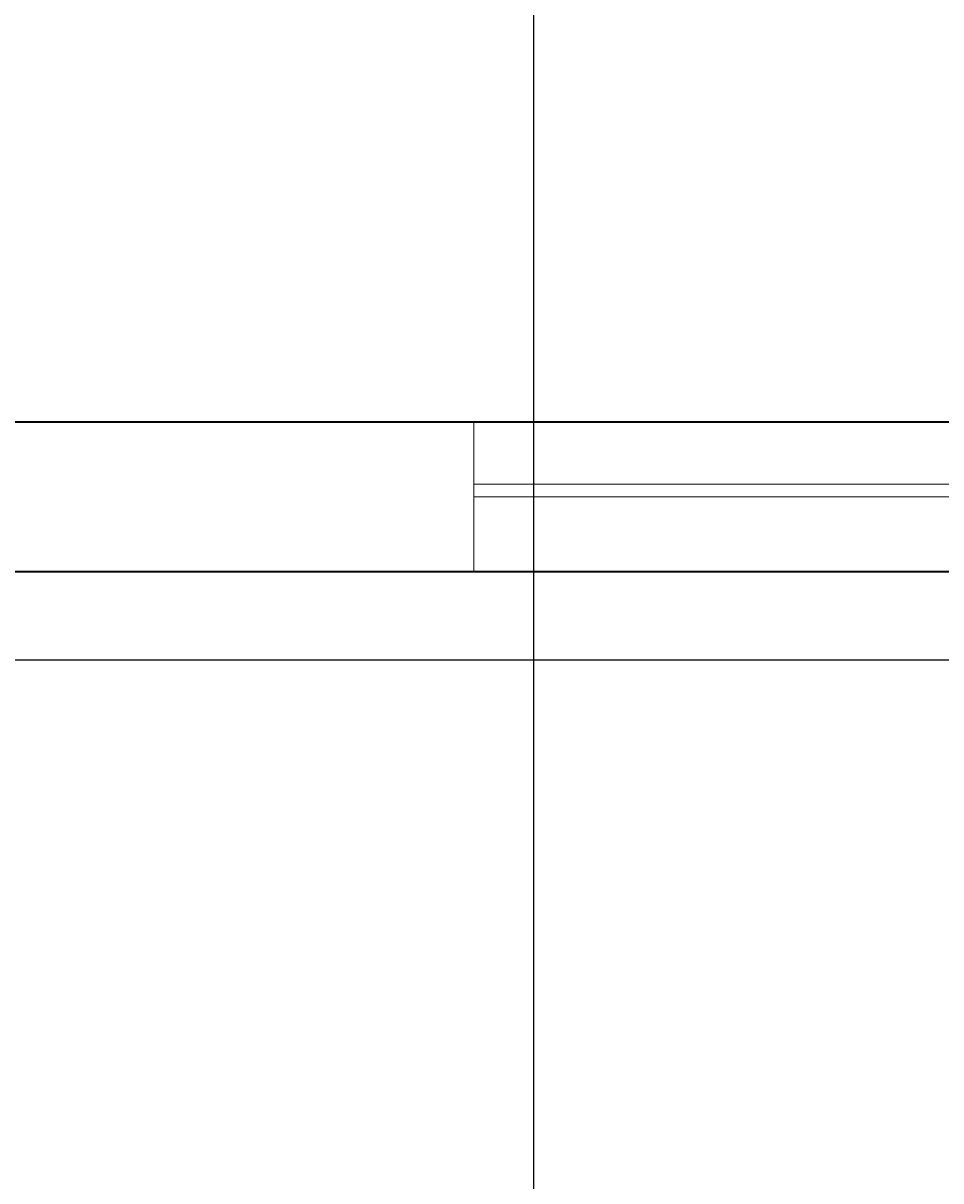
# Model space of a CAD drawing. Units: inches. Extents: x -61 to 1599, y -1316 to 257.
# Tile 51 of 204: x 185 to 240, y -478 to -408. Entities that reach past the tile are written whole.
import ezdxf

# ---------------------------------------------------------------- set-up
doc = ezdxf.new("R2010")
doc.units = ezdxf.units.IN
doc.header["$MEASUREMENT"] = 0
for name, color, linetype, lineweight in [('A-ANNO-DIMS', 2, 'Continuous', 18), ('WALLS', 4, 'Continuous', 35), ('WINDOWS', 220, 'Continuous', 18)]:
    doc.layers.add(name, color=color, linetype=linetype, lineweight=lineweight)
doc.styles.get("Standard").update_dxf_attribs({"font": 'arial.ttf'})
doc.dimstyles.get("Standard").update_dxf_attribs({"dimtxt": 0.18, "dimasz": 0.18, "dimexe": 0.18, "dimexo": 0.0625, "dimgap": 0.09, "dimtad": 0, "dimtih": 1, "dimtoh": 1, "dimdec": 0, "dimzin": 0, "dimdsep": 46, "dimlunit": 3, "dimtxsty": 'Standard', "dimcen": 0.09, "dimadec": 0, "dimazin": 0, "dimtfac": 1, "dimtdec": 0, "dimtofl": 0, "dimtmove": 0, "dimatfit": 3, "dimfxl": 1, "dimtolj": 1, "dimtzin": 0, "dimarcsym": 0})

# ---------------------------------------------------------------- blocks, each defined once
blk = doc.blocks.new('WIN-36IN-2')
for p, q in [((0, 9), (0, 0)), ((36, 9), (36, 0)), ((0, 5.262), (36, 5.262)), ((0, 4.5), (36, 4.5)), ((0, 4.5), (36, 4.5))]:
    blk.add_line(p, q)
blk = doc.blocks.new('*D687')
at = {"layer": 'A-ANNO-DIMS', "color": 0, "lineweight": -2, "transparency": 16777216}
for p, q in [((289.418, 181.677), (-61.077, 181.677)), ((-60.897, 181.497), (-60.897, -528.952)), ((-60.897, -1239.765), (-60.897, -529.316)), ((319.64, -1239.945), (-61.077, -1239.945))]:
    blk.add_line(p, q, dxfattribs=at)
at = {"layer": 'A-ANNO-DIMS', "color": 0, "transparency": 16777216}
for points in [[(-60.927, 181.497), (-60.867, 181.497), (-60.897, 181.677)], [(-60.927, -1239.765), (-60.867, -1239.765), (-60.897, -1239.945)]]:
    blk.add_solid(points, dxfattribs=at)
at = {"layer": 'DEFPOINTS', "color": 0, "transparency": 16777216}
for p in [(289.481, 181.677), (-60.897, -1239.945), (319.703, -1239.945)]:
    blk.add_point(p, dxfattribs=at)
at = {"layer": 'A-ANNO-DIMS', "color": 0, "transparency": 16777216, "insert": (-60.897, -529.134), "char_height": 0.18, "attachment_point": 5}
blk.add_mtext('\\A1;1421.6', dxfattribs=at)
blk = doc.blocks.new('*D699')
at = {"layer": 'A-ANNO-DIMS', "color": 0, "lineweight": -2, "transparency": 16777216}
for p, q in [((835.64, -167.169), (-61.077, -167.169)), ((-60.897, -167.349), (-60.897, -306.726)), ((-60.897, -446.466), (-60.897, -307.09)), ((841.64, -446.646), (-61.077, -446.646))]:
    blk.add_line(p, q, dxfattribs=at)
at = {"layer": 'A-ANNO-DIMS', "color": 0, "transparency": 16777216}
for points in [[(-60.927, -167.349), (-60.867, -167.349), (-60.897, -167.169)], [(-60.927, -446.466), (-60.867, -446.466), (-60.897, -446.646)]]:
    blk.add_solid(points, dxfattribs=at)
at = {"layer": 'DEFPOINTS', "color": 0, "transparency": 16777216}
for p in [(835.703, -167.169), (-60.897, -446.646), (841.703, -446.646)]:
    blk.add_point(p, dxfattribs=at)
at = {"layer": 'A-ANNO-DIMS', "color": 0, "transparency": 16777216, "insert": (-60.897, -306.908), "char_height": 0.18, "attachment_point": 5}
blk.add_mtext('\\A1;279.5', dxfattribs=at)
blk = doc.blocks.new('*D701')
at = {"layer": 'A-ANNO-DIMS', "color": 0, "lineweight": -2, "transparency": 16777216}
for p, q in [((215.752, -616.882), (215.752, 257.457)), ((215.932, 257.277), (233.924, 257.277)), ((252.702, 257.277), (234.711, 257.277)), ((252.882, -616.882), (252.882, 257.457))]:
    blk.add_line(p, q, dxfattribs=at)
at = {"layer": 'A-ANNO-DIMS', "color": 0, "transparency": 16777216}
for points in [[(215.932, 257.307), (215.932, 257.247), (215.752, 257.277)], [(252.702, 257.307), (252.702, 257.247), (252.882, 257.277)]]:
    blk.add_solid(points, dxfattribs=at)
at = {"layer": 'DEFPOINTS', "color": 0, "transparency": 16777216}
for p in [(252.882, 257.277), (215.752, -616.945), (252.882, -616.945)]:
    blk.add_point(p, dxfattribs=at)
at = {"layer": 'A-ANNO-DIMS', "color": 0, "transparency": 16777216, "insert": (234.317, 257.277), "char_height": 0.18, "attachment_point": 5}
blk.add_mtext('\\A1;37.13', dxfattribs=at)

msp = doc.modelspace()

# ---------------------------------------------------------------- linework, layer by layer
at = {"layer": 'WALLS'}
for p, q in [((87.7028, -432.3229), (237.7028, -432.3229)), ((237.7028, -432.3229), (259.7028, -432.3229)), ((14.7028, -441.3229), (237.7028, -441.3229)), ((237.7028, -441.3229), (319.7028, -441.3229))]:
    msp.add_line(p, q, dxfattribs=at)

# ---------------------------------------------------------------- block references
at = {"layer": 'WINDOWS'}
msp.add_blockref('WIN-36IN-2', (212.158, -441.323), dxfattribs=at)

# ---------------------------------------------------------------- dimensions: what is measured, and where the dimension line sits
at = {"layer": 'A-ANNO-DIMS'}
dim = msp.add_linear_dim(base=(252.8825, 257.2771), p1=(215.7521, -616.9446), p2=(252.8825, -616.9446), dimstyle='Standard', override={"dimdec": 2, "dimlfac": 1, "dimrnd": 0, "dimzin": 0, "dimdsep": 46, "dimlunit": 2}, dxfattribs=at)
dim.commit()
dim.dimension.update_dxf_attribs({"geometry": '*D701', "text_midpoint": (234.3173, 257.2771)})
for base, p1, p2, picture, middle in [((-60.8972, -1239.9446), (289.4807, 181.6771), (319.7028, -1239.9446), '*D687', (-60.8972, -529.1337)), ((-60.8972, -446.6462), (835.7028, -167.169), (841.7028, -446.6462), '*D699', (-60.8972, -306.9076))]:
    dim = msp.add_linear_dim(base=base, p1=p1, p2=p2, angle=90, dimstyle='Standard', override={"dimdec": 1, "dimlfac": 1, "dimrnd": 0, "dimzin": 0, "dimdsep": 46, "dimlunit": 2}, dxfattribs=at)
    dim.commit()
    dim.dimension.update_dxf_attribs({"geometry": picture, "text_midpoint": middle})

doc.saveas('drawing.dxf')
